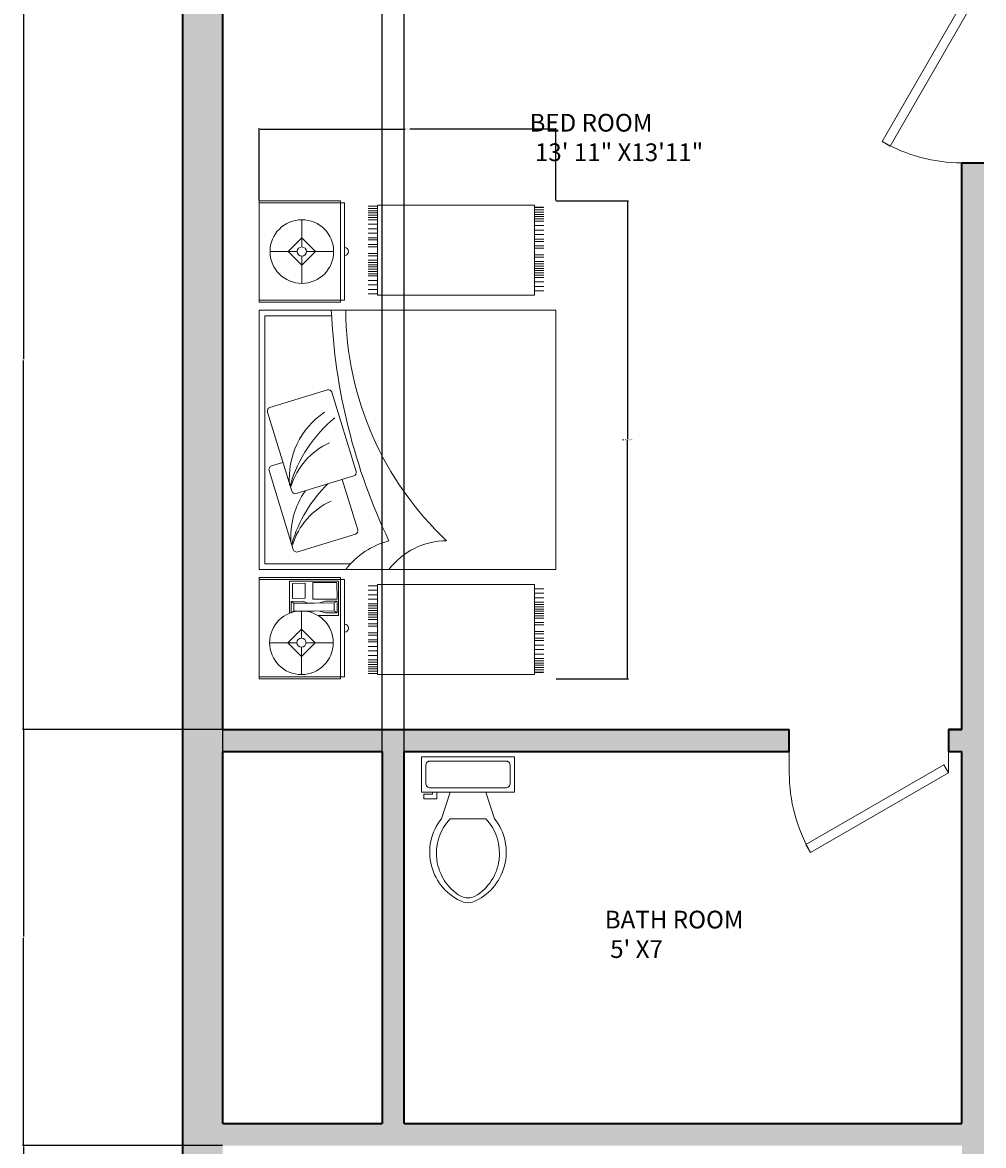
# Model space of a CAD drawing. Units: inches. Extents: x -29 to 404, y -32 to 761.
# Tile 3 of 5: x -29 to 189, y 193 to 447. Entities that reach past the tile are written whole.
import ezdxf

# ---------------------------------------------------------------- set-up
doc = ezdxf.new("R2010")
doc.units = ezdxf.units.IN
doc.header["$MEASUREMENT"] = 0
for name, color, linetype, lineweight in [('A-ANNO-DIMS', 2, 'Continuous', 18), ('A-AREA-IDEN', 7, 'Continuous', 18), ('A-FLOR-FIXT', 9, 'Continuous', 18), ('A-FURN', 8, 'Continuous', 18), ('A-WALL', 7, 'Continuous', 35), ('doors', 40, 'Continuous', 20)]:
    doc.layers.add(name, color=color, linetype=linetype, lineweight=lineweight)
doc.layers.add('A-WALL-PATT', color=251, linetype='Continuous', lineweight=13, true_color=0x636466)
doc.styles.get("Standard").update_dxf_attribs({"font": 'arial.ttf'})
doc.dimstyles.get("Standard").update_dxf_attribs({"dimtxt": 0.18, "dimasz": 0.18, "dimexe": 0.18, "dimexo": 0.0625, "dimgap": 0.09, "dimtad": 0, "dimtih": 1, "dimtoh": 1, "dimdec": 4, "dimzin": 0, "dimdsep": 46, "dimtxsty": 'Standard', "dimcen": 0.09, "dimadec": 0, "dimazin": 0, "dimtfac": 1, "dimtdec": 4, "dimtofl": 0, "dimtmove": 0, "dimatfit": 3, "dimfxl": 1, "dimtolj": 1, "dimtzin": 0, "dimarcsym": 0})

# ---------------------------------------------------------------- blocks, each defined once
blk = doc.blocks.new('3')
for p, q in [((185.8665, 224.6766), (185.8665, 225.2363)), ((185.8665, 225.2363), (186.566, 225.2363)), ((185.8805, 224.6487), (185.8805, 225.2363)), ((186.552, 225.2363), (186.552, 224.6487)), ((186.566, 225.2363), (186.566, 224.6766)), ((186.6199, 225.2363), (186.6199, 224.6399)), ((188.4089, 225.2363), (186.6199, 225.2363)), ((188.4089, 224.7393), (188.4089, 225.2363)), ((188.4627, 225.2363), (188.4627, 224.6766)), ((189.1623, 225.2363), (188.4627, 225.2363)), ((188.4767, 225.2363), (188.4767, 224.6486)), ((189.1483, 224.6486), (189.1483, 225.2363)), ((189.1623, 224.6766), (189.1623, 225.2363)), ((186.1157, 225.1643), (186.1157, 224.9763)), ((187.3034, 225.1683), (186.7581, 225.0015)), ((187.7059, 225.1793), (187.1607, 225.0124)), ((187.3344, 225.1518), (187.3586, 225.073)), ((187.737, 225.1628), (187.8585, 224.7657)), ((188.8125, 225.1618), (188.8125, 224.9738)), ((186.0216, 224.9449), (186.1157, 225.0389)), ((186.1157, 225.0389), (186.2097, 224.9449)), ((186.5397, 225.0274), (186.3193, 225.0266)), ((186.3215, 225.0167), (186.4008, 225.017)), ((186.3334, 224.9969), (186.3215, 225.0167)), ((186.3334, 224.9969), (186.389, 224.9971)), ((186.334, 224.858), (186.3334, 224.9969)), ((186.4008, 225.017), (186.389, 224.9971)), ((186.3895, 224.8582), (186.389, 224.9971)), ((186.4008, 225.017), (186.4011, 224.9376)), ((186.5409, 224.6901), (186.5397, 225.0274)), ((188.8125, 225.0365), (188.7185, 224.9424)), ((188.9065, 224.9424), (188.8125, 225.0365)), ((186.0843, 224.9449), (185.8963, 224.9449)), ((186.1157, 224.8509), (186.0216, 224.9449)), ((186.2097, 224.9449), (186.1157, 224.8509)), ((186.1157, 224.9136), (186.1157, 224.7256)), ((186.147, 224.9449), (186.335, 224.9449)), ((186.4011, 224.9376), (186.3894, 224.8979)), ((186.7416, 224.9704), (186.8631, 224.5734)), ((187.1442, 224.9814), (187.2657, 224.5843)), ((188.7812, 224.9424), (188.5931, 224.9424)), ((188.7185, 224.9424), (188.8125, 224.8484)), ((188.8125, 224.8484), (188.9065, 224.9424)), ((188.8125, 224.9111), (188.8125, 224.723)), ((188.8438, 224.9424), (189.0319, 224.9424)), ((186.3023, 224.8297), (186.3029, 224.6892)), ((186.3314, 224.9055), (186.3338, 224.8977)), ((186.334, 224.858), (186.3345, 224.7191)), ((186.3895, 224.8582), (186.39, 224.7193)), ((186.3224, 224.7786), (186.3341, 224.8183)), ((186.3227, 224.6992), (186.3224, 224.7786)), ((186.4017, 224.7789), (186.3897, 224.8185)), ((186.402, 224.6995), (186.4017, 224.7789)), ((186.566, 224.6766), (185.8665, 224.6766)), ((186.3029, 224.6892), (186.5409, 224.6901)), ((186.3345, 224.7191), (186.3227, 224.6992)), ((186.3227, 224.6992), (186.402, 224.6995)), ((186.3345, 224.7191), (186.39, 224.7193)), ((186.402, 224.6995), (186.39, 224.7193)), ((187.842, 224.7347), (187.2967, 224.5678)), ((188.4089, 224.7393), (188.4089, 223.1907)), ((188.4627, 224.6766), (189.1623, 224.6766)), ((186.552, 224.6487), (185.8805, 224.6487)), ((186.6199, 224.6399), (186.6199, 223.1907)), ((187.2416, 224.6632), (186.8942, 224.5569)), ((188.4767, 224.6486), (189.1483, 224.6486)), ((185.904, 224.4849, -0.9094), (185.904, 224.4204, -0.9094)), ((185.9195, 224.4849, -0.9094), (185.9195, 224.4204, -0.9094)), ((185.9195, 224.4849, -0.9094), (185.9195, 224.4204, -0.9094)), ((185.935, 224.4849, -0.9094), (185.935, 224.4204, -0.9094)), ((185.9505, 224.4849, -0.9094), (185.9505, 224.4204, -0.9094)), ((185.966, 224.4849, -0.9094), (185.966, 224.4204, -0.9094)), ((185.9815, 224.4849, -0.9094), (185.9815, 224.4204, -0.9094)), ((185.997, 224.4849, -0.9094), (185.997, 224.4204, -0.9094)), ((186.028, 224.4849, -0.9094), (186.028, 224.4204, -0.9094)), ((186.059, 224.4849, -0.9094), (186.059, 224.4204, -0.9094)), ((186.09, 224.4849, -0.9094), (186.09, 224.4204, -0.9094)), ((186.09, 224.4849, -0.9094), (186.09, 224.4204, -0.9094)), ((186.121, 224.4849, -0.9094), (186.121, 224.4204, -0.9094)), ((186.1365, 224.4849, -0.9094), (186.1365, 224.4204, -0.9094)), ((186.1675, 224.4849, -0.9094), (186.1675, 224.4204, -0.9094)), ((186.183, 224.4849, -0.9094), (186.183, 224.4204, -0.9094)), ((186.2295, 224.4849, -0.9094), (186.2295, 224.4204, -0.9094)), ((186.245, 224.4849, -0.9094), (186.245, 224.4204, -0.9094)), ((186.276, 224.4849, -0.9094), (186.276, 224.4204, -0.9094)), ((186.2915, 224.4849, -0.9094), (186.2915, 224.4204, -0.9094)), ((186.307, 224.4849, -0.9094), (186.307, 224.4204, -0.9094)), ((186.3225, 224.4849, -0.9094), (186.3225, 224.4204, -0.9094)), ((186.338, 224.4849, -0.9094), (186.338, 224.4204, -0.9094)), ((186.3535, 224.4849, -0.9094), (186.3535, 224.4204, -0.9094)), ((186.369, 224.4849, -0.9094), (186.369, 224.4204, -0.9094)), ((186.3845, 224.4849, -0.9094), (186.3845, 224.4204, -0.9094)), ((186.4155, 224.4849, -0.9094), (186.4155, 224.4204, -0.9094)), ((186.4465, 224.4849, -0.9094), (186.4465, 224.4204, -0.9094)), ((186.4775, 224.4849, -0.9094), (186.4775, 224.4204, -0.9094)), ((186.5085, 224.4849, -0.9094), (186.5085, 224.4204, -0.9094)), ((188.5202, 224.4849, -0.9094), (188.5202, 224.4204, -0.9094)), ((188.5512, 224.4849, -0.9094), (188.5512, 224.4204, -0.9094)), ((188.5822, 224.4849, -0.9094), (188.5822, 224.4204, -0.9094)), ((188.6132, 224.4849, -0.9094), (188.6132, 224.4204, -0.9094)), ((188.6442, 224.4849, -0.9094), (188.6442, 224.4204, -0.9094)), ((188.6597, 224.4849, -0.9094), (188.6597, 224.4204, -0.9094)), ((188.6752, 224.4849, -0.9094), (188.6752, 224.4204, -0.9094)), ((188.6907, 224.4849, -0.9094), (188.6907, 224.4204, -0.9094)), ((188.7062, 224.4849, -0.9094), (188.7062, 224.4204, -0.9094)), ((188.7217, 224.4849, -0.9094), (188.7217, 224.4204, -0.9094)), ((188.7372, 224.4849, -0.9094), (188.7372, 224.4204, -0.9094)), ((188.7527, 224.4849, -0.9094), (188.7527, 224.4204, -0.9094)), ((188.7837, 224.4849, -0.9094), (188.7837, 224.4204, -0.9094)), ((188.7992, 224.4849, -0.9094), (188.7992, 224.4204, -0.9094)), ((188.8457, 224.4849, -0.9094), (188.8457, 224.4204, -0.9094)), ((188.8612, 224.4849, -0.9094), (188.8612, 224.4204, -0.9094)), ((188.8922, 224.4849, -0.9094), (188.8922, 224.4204, -0.9094)), ((188.9077, 224.4849, -0.9094), (188.9077, 224.4204, -0.9094)), ((188.9387, 224.4849, -0.9094), (188.9387, 224.4204, -0.9094)), ((188.9387, 224.4849, -0.9094), (188.9387, 224.4204, -0.9094)), ((188.9697, 224.4849, -0.9094), (188.9697, 224.4204, -0.9094)), ((189.0007, 224.4849, -0.9094), (189.0007, 224.4204, -0.9094)), ((189.0317, 224.4849, -0.9094), (189.0317, 224.4204, -0.9094)), ((189.0472, 224.4849, -0.9094), (189.0472, 224.4204, -0.9094)), ((189.0627, 224.4849, -0.9094), (189.0627, 224.4204, -0.9094)), ((189.0782, 224.4849, -0.9094), (189.0782, 224.4204, -0.9094)), ((189.0937, 224.4849, -0.9094), (189.0937, 224.4204, -0.9094)), ((189.1092, 224.4849, -0.9094), (189.1092, 224.4204, -0.9094)), ((189.1092, 224.4849, -0.9094), (189.1092, 224.4204, -0.9094)), ((189.1247, 224.4849, -0.9094), (189.1247, 224.4204, -0.9094)), ((185.8974, 224.4204, -0.9094), (185.8974, 223.3378, -0.9094)), ((185.8974, 224.4204, -0.9094), (186.5174, 224.4204, -0.9094)), ((186.5174, 224.4204, -0.9094), (186.5174, 223.3378, -0.9094)), ((189.1313, 224.4204, -0.9094), (188.5113, 224.4204, -0.9094)), ((188.5113, 224.4204, -0.9094), (188.5113, 223.3378, -0.9094)), ((189.1313, 224.4204, -0.9094), (189.1313, 223.3378, -0.9094)), ((185.8974, 223.3378, -0.9094), (186.5174, 223.3378, -0.9094)), ((185.9114, 223.3378, -0.9094), (185.9114, 223.2789, -0.9094)), ((185.9114, 223.3378, -0.9094), (185.9114, 223.2789, -0.9094)), ((185.9114, 223.3378, -0.9094), (185.9114, 223.2789, -0.9094)), ((185.9138, 223.3378, -0.9094), (185.9138, 223.2732, -0.9094)), ((185.9293, 223.3378, -0.9094), (185.9293, 223.2732, -0.9094)), ((185.9293, 223.3378, -0.9094), (185.9293, 223.2732, -0.9094)), ((185.9448, 223.3378, -0.9094), (185.9448, 223.2732, -0.9094)), ((185.9603, 223.3378, -0.9094), (185.9603, 223.2732, -0.9094)), ((185.9758, 223.3378, -0.9094), (185.9758, 223.2732, -0.9094)), ((185.9913, 223.3378, -0.9094), (185.9913, 223.2732, -0.9094)), ((186.0068, 223.3378, -0.9094), (186.0068, 223.2732, -0.9094)), ((186.0378, 223.3378, -0.9094), (186.0378, 223.2732, -0.9094)), ((186.0688, 223.3378, -0.9094), (186.0688, 223.2732, -0.9094)), ((186.0998, 223.3378, -0.9094), (186.0998, 223.2732, -0.9094)), ((186.0998, 223.3378, -0.9094), (186.0998, 223.2732, -0.9094)), ((186.1308, 223.3378, -0.9094), (186.1308, 223.2732, -0.9094)), ((186.1463, 223.3378, -0.9094), (186.1463, 223.2732, -0.9094)), ((186.1773, 223.3378, -0.9094), (186.1773, 223.2732, -0.9094)), ((186.1928, 223.3378, -0.9094), (186.1928, 223.2732, -0.9094)), ((186.2393, 223.3378, -0.9094), (186.2393, 223.2732, -0.9094)), ((186.2548, 223.3378, -0.9094), (186.2548, 223.2732, -0.9094)), ((186.2858, 223.3378, -0.9094), (186.2858, 223.2732, -0.9094)), ((186.3013, 223.3378, -0.9094), (186.3013, 223.2732, -0.9094)), ((186.3168, 223.3378, -0.9094), (186.3168, 223.2732, -0.9094)), ((186.3323, 223.3378, -0.9094), (186.3323, 223.2732, -0.9094)), ((186.3478, 223.3378, -0.9094), (186.3478, 223.2732, -0.9094)), ((186.3633, 223.3378, -0.9094), (186.3633, 223.2732, -0.9094)), ((186.3788, 223.3378, -0.9094), (186.3788, 223.2732, -0.9094)), ((186.3943, 223.3378, -0.9094), (186.3943, 223.2732, -0.9094)), ((186.4253, 223.3378, -0.9094), (186.4253, 223.2732, -0.9094)), ((186.4563, 223.3378, -0.9094), (186.4563, 223.2732, -0.9094)), ((186.4873, 223.3378, -0.9094), (186.4873, 223.2732, -0.9094)), ((189.1313, 223.3378, -0.9094), (188.5113, 223.3378, -0.9094)), ((188.5414, 223.3378, -0.9094), (188.5414, 223.2732, -0.9094)), ((188.5724, 223.3378, -0.9094), (188.5724, 223.2732, -0.9094)), ((188.6034, 223.3378, -0.9094), (188.6034, 223.2732, -0.9094)), ((188.6344, 223.3378, -0.9094), (188.6344, 223.2732, -0.9094)), ((188.6499, 223.3378, -0.9094), (188.6499, 223.2732, -0.9094)), ((188.6654, 223.3378, -0.9094), (188.6654, 223.2732, -0.9094)), ((188.6809, 223.3378, -0.9094), (188.6809, 223.2732, -0.9094)), ((188.6964, 223.3378, -0.9094), (188.6964, 223.2732, -0.9094)), ((188.7119, 223.3378, -0.9094), (188.7119, 223.2732, -0.9094)), ((188.7274, 223.3378, -0.9094), (188.7274, 223.2732, -0.9094)), ((188.7429, 223.3378, -0.9094), (188.7429, 223.2732, -0.9094)), ((188.7739, 223.3378, -0.9094), (188.7739, 223.2732, -0.9094)), ((188.7894, 223.3378, -0.9094), (188.7894, 223.2732, -0.9094)), ((188.8359, 223.3378, -0.9094), (188.8359, 223.2732, -0.9094)), ((188.8514, 223.3378, -0.9094), (188.8514, 223.2732, -0.9094)), ((188.8824, 223.3378, -0.9094), (188.8824, 223.2732, -0.9094)), ((188.8979, 223.3378, -0.9094), (188.8979, 223.2732, -0.9094)), ((188.9289, 223.3378, -0.9094), (188.9289, 223.2732, -0.9094)), ((188.9289, 223.3378, -0.9094), (188.9289, 223.2732, -0.9094)), ((188.9599, 223.3378, -0.9094), (188.9599, 223.2732, -0.9094)), ((188.9909, 223.3378, -0.9094), (188.9909, 223.2732, -0.9094)), ((189.022, 223.3378, -0.9094), (189.022, 223.2732, -0.9094)), ((189.0375, 223.3378, -0.9094), (189.0375, 223.2732, -0.9094)), ((189.053, 223.3378, -0.9094), (189.053, 223.2732, -0.9094)), ((189.0685, 223.3378, -0.9094), (189.0685, 223.2732, -0.9094)), ((189.084, 223.3378, -0.9094), (189.084, 223.2732, -0.9094)), ((189.0995, 223.3378, -0.9094), (189.0995, 223.2732, -0.9094)), ((189.0995, 223.3378, -0.9094), (189.0995, 223.2732, -0.9094)), ((189.115, 223.3378, -0.9094), (189.115, 223.2732, -0.9094)), ((189.1173, 223.3378, -0.9094), (189.1173, 223.2789, -0.9094)), ((189.1173, 223.3378, -0.9094), (189.1173, 223.2789, -0.9094)), ((189.1173, 223.3378, -0.9094), (189.1173, 223.2789, -0.9094)), ((186.6199, 223.1907), (188.4089, 223.1907))]:
    blk.add_line(p, q)
blk.add_lwpolyline([(188.3691, 224.7374), (188.3691, 225.1965), (186.6596, 225.1965), (186.6596, 224.606)])
for points in [[(186.4217, 225.0072), (186.422, 224.9199), (186.5252, 224.9202), (186.5249, 225.0075)], [(186.4153, 224.8663), (186.4159, 224.6996), (186.531, 224.7), (186.5304, 224.8667)]]:
    blk.add_lwpolyline(points, close=True)
for points in [[(186.6199, 224.6399, -0.162278), (186.8186, 224.3418, -0.100664), (188.4089, 224.7393, -0.100664)], [(186.6199, 224.3418, -0.236068), (186.8186, 223.9442, -0.205258), (188.4089, 224.6399, -0.205258)]]:
    blk.add_lwpolyline(points, format="xyb")
for centre, radius in [((186.1157, 224.9449), 0.2194), ((188.8125, 224.9424), 0.2194), ((186.1157, 224.9449), 0.0313), ((188.8125, 224.9424), 0.0313)]:
    blk.add_circle(centre, radius)
for centre, radius, start, end in [((187.3107, 225.1446), 0.0248, 17.0142, 107.0142), ((187.7132, 225.1555), 0.0248, 17.0142, 107.0142), ((186.7654, 224.9777), 0.0248, 107.0142, 197.0142), ((186.6474, 224.5408), 0.4873, 24.22087, 73.06906), ((186.8477, 224.4712), 0.5468, 54.68511, 95.16051), ((186.5359, 224.1054), 0.9426, 44.27274, 73.71889), ((187.1679, 224.9887), 0.0248, 107.0142, 197.0142), ((187.0499, 224.5517), 0.4873, 24.22087, 73.06906), ((187.2502, 224.4821), 0.5468, 33.78007, 95.16051), ((186.9385, 224.1164), 0.9426, 39.40233, 73.71889), ((187.8347, 224.7585), 0.0248, 287.0142, 17.0142), ((186.2163, 224.6487), 0.028, 180, 0), ((188.8125, 224.6486), 0.028, 180, 0), ((186.8869, 224.5806), 0.0248, 197.0142, 287.0142), ((187.2894, 224.5916), 0.0248, 197.0142, 287.0142)]:
    blk.add_arc(centre, radius, start, end)
blk = doc.blocks.new('Toilet - top')
for p, q in [((9.5, -6), (9.5, -2)), ((-10, -8.5), (-8, -8.5)), ((-10, -9.5), (-10, -8.5)), ((-7, -9.5), (-10, -9.5)), ((-8, -8.5), (-8, -8)), ((-7, -8), (-7, -9.5)), ((-4, -8), (-6, -14)), ((4, -8), (6, -14)), ((4, -14), (-4, -14))]:
    blk.add_line(p, q)
blk.add_lwpolyline([(10.5, -8), (10.5, 0), (-10.5, 0), (-10.5, -8)], close=True)
for points in [[(-9.5, -2), (-9.5, -6)], [(8.5, -1), (-8.5, -1)], [(-8.5, -7), (8.5, -7)]]:
    blk.add_lwpolyline(points)
for centre, radius, start, end in [((-8.62, -1.88), 0.884, 81.8699, 188.1301), ((8.62, -1.88), 0.884, 351.8699, 98.1301), ((-8.62, -6.12), 0.884, 171.8699, 278.1301), ((8.62, -6.12), 0.884, 261.8699, 8.1301), ((3.52, -21.58), 12.17, 141.4691, 247.9714), ((4.2, -21.82), 11.33, 136.3677, 238.9468), ((-3.52, -21.58), 12.17, 292.0284, 38.5307), ((-4.2, -21.82), 11.33, 301.053, 43.6321), ((0, -27.88), 4, 245.7318, 294.2682), ((0, -29), 4, 254.8605, 285.1395)]:
    blk.add_arc(centre, radius, start, end)
blk = doc.blocks.new('*U6')
for p, q in [((0, 0), (0, -100)), ((750, 0), (750, -100))]:
    blk.add_line(p, q)
blk.add_lwpolyline([(0, 0), (649.5, 375), (671.4, 337.1), (21.9, -37.9)], close=True)
blk.add_arc((0, 0), 750, 0, 30)
blk = doc.blocks.new('*U7')
for p, q in [((0, 0), (0, 100)), ((750, 0), (750, 100))]:
    blk.add_line(p, q)
blk.add_lwpolyline([(0, 0), (649.5, -375), (671.4, -337.1), (21.9, 37.9)], close=True)
blk.add_arc((0, 0), 750, 330, 0)
blk = doc.blocks.new('*D13')
at = {"layer": 'A-ANNO-DIMS', "color": 0, "lineweight": -2, "transparency": 16777216}
for p, q in [((92.01, 406.85), (108.33, 406.85)), ((108.15, 406.67), (108.15, 353.04)), ((108.15, 299.03), (108.15, 352.67)), ((92.01, 298.85), (108.33, 298.85))]:
    blk.add_line(p, q, dxfattribs=at)
at = {"layer": 'A-ANNO-DIMS', "color": 0, "transparency": 16777216}
for points in [[(108.12, 406.67), (108.18, 406.67), (108.15, 406.85)], [(108.12, 299.03), (108.18, 299.03), (108.15, 298.85)]]:
    blk.add_solid(points, dxfattribs=at)
at = {"layer": 'Defpoints', "color": 0, "transparency": 16777216}
for p in [(91.95, 406.85), (108.15, 406.85), (91.95, 298.85)]:
    blk.add_point(p, dxfattribs=at)
at = {"layer": 'A-ANNO-DIMS', "color": 0, "transparency": 16777216, "insert": (108.15, 352.85), "char_height": 0.18, "attachment_point": 5}
blk.add_mtext('\\A1;BED GROUP 108 TYP.', dxfattribs=at)
blk = doc.blocks.new('*D14')
at = {"layer": 'A-ANNO-DIMS', "color": 0, "lineweight": -2, "transparency": 16777216}
for p, q in [((24.92, 406.91), (24.92, 423.23)), ((25.1, 423.05), (57.91, 423.05)), ((91.77, 423.05), (58.96, 423.05)), ((91.95, 406.91), (91.95, 423.23))]:
    blk.add_line(p, q, dxfattribs=at)
at = {"layer": 'A-ANNO-DIMS', "color": 0, "transparency": 16777216}
for points in [[(25.1, 423.08), (25.1, 423.02), (24.92, 423.05)], [(91.77, 423.08), (91.77, 423.02), (91.95, 423.05)]]:
    blk.add_solid(points, dxfattribs=at)
at = {"layer": 'Defpoints', "color": 0, "transparency": 16777216}
for p in [(24.92, 423.05), (24.92, 406.85), (91.95, 406.85)]:
    blk.add_point(p, dxfattribs=at)
at = {"layer": 'A-ANNO-DIMS', "color": 0, "transparency": 16777216, "insert": (58.44, 423.05), "char_height": 0.18, "attachment_point": 5}
blk.add_mtext('\\A1;67 TYP.', dxfattribs=at)
blk = doc.blocks.new('*D33')
at = {"layer": 'A-ANNO-DIMS', "color": 0, "lineweight": -2, "transparency": 16777216}
for p, q in [((16.62, 193.43), (-28.55, 193.43)), ((-28.37, 193.25), (-28.37, 99.12)), ((-28.37, 4.61), (-28.37, 98.75)), ((7.62, 4.43), (-28.55, 4.43))]:
    blk.add_line(p, q, dxfattribs=at)
at = {"layer": 'A-ANNO-DIMS', "color": 0, "transparency": 16777216}
for points in [[(-28.4, 193.25), (-28.34, 193.25), (-28.37, 193.43)], [(-28.4, 4.61), (-28.34, 4.61), (-28.37, 4.43)]]:
    blk.add_solid(points, dxfattribs=at)
at = {"layer": 'Defpoints', "color": 0, "transparency": 16777216}
for p in [(-28.37, 193.43), (16.68, 193.43), (7.68, 4.43)]:
    blk.add_point(p, dxfattribs=at)
at = {"layer": 'A-ANNO-DIMS', "color": 0, "transparency": 16777216, "insert": (-28.37, 98.93), "char_height": 0.18, "attachment_point": 5}
blk.add_mtext('\\A1;189', dxfattribs=at)
blk = doc.blocks.new('*D34')
at = {"layer": 'A-ANNO-DIMS', "color": 0, "lineweight": -2, "transparency": 16777216}
for p, q in [((16.62, 287.43), (-28.55, 287.43)), ((-28.37, 287.25), (-28.37, 240.62)), ((-28.37, 193.61), (-28.37, 240.25)), ((16.62, 193.43), (-28.55, 193.43))]:
    blk.add_line(p, q, dxfattribs=at)
at = {"layer": 'A-ANNO-DIMS', "color": 0, "transparency": 16777216}
for points in [[(-28.4, 287.25), (-28.34, 287.25), (-28.37, 287.43)], [(-28.4, 193.61), (-28.34, 193.61), (-28.37, 193.43)]]:
    blk.add_solid(points, dxfattribs=at)
at = {"layer": 'Defpoints', "color": 0, "transparency": 16777216}
for p in [(-28.37, 287.43), (16.68, 287.43), (16.68, 193.43)]:
    blk.add_point(p, dxfattribs=at)
at = {"layer": 'A-ANNO-DIMS', "color": 0, "transparency": 16777216, "insert": (-28.37, 240.43), "char_height": 0.18, "attachment_point": 5}
blk.add_mtext('\\A1;94', dxfattribs=at)
blk = doc.blocks.new('*D35')
at = {"layer": 'A-ANNO-DIMS', "color": 0, "lineweight": -2, "transparency": 16777216}
for p, q in [((16.62, 454.43), (-28.55, 454.43)), ((-28.37, 454.25), (-28.37, 371.12)), ((-28.37, 287.61), (-28.37, 370.75)), ((16.62, 287.43), (-28.55, 287.43))]:
    blk.add_line(p, q, dxfattribs=at)
at = {"layer": 'A-ANNO-DIMS', "color": 0, "transparency": 16777216}
for points in [[(-28.4, 454.25), (-28.34, 454.25), (-28.37, 454.43)], [(-28.4, 287.61), (-28.34, 287.61), (-28.37, 287.43)]]:
    blk.add_solid(points, dxfattribs=at)
at = {"layer": 'Defpoints', "color": 0, "transparency": 16777216}
for p in [(-28.37, 454.43), (16.68, 454.43), (16.68, 287.43)]:
    blk.add_point(p, dxfattribs=at)
at = {"layer": 'A-ANNO-DIMS', "color": 0, "transparency": 16777216, "insert": (-28.37, 370.93), "char_height": 0.18, "attachment_point": 5}
blk.add_mtext('\\A1;167', dxfattribs=at)
blk = doc.blocks.new('*D59')
at = {"layer": 'A-ANNO-DIMS', "color": 0, "lineweight": -2, "transparency": 16777216}
for p, q in [((16.68, 198.5), (16.68, 760.66)), ((16.86, 760.48), (34.46, 760.48)), ((52.5, 760.48), (34.9, 760.48)), ((52.68, 198.5), (52.68, 760.66))]:
    blk.add_line(p, q, dxfattribs=at)
at = {"layer": 'A-ANNO-DIMS', "color": 0, "transparency": 16777216}
for points in [[(16.86, 760.51), (16.86, 760.45), (16.68, 760.48)], [(52.5, 760.51), (52.5, 760.45), (52.68, 760.48)]]:
    blk.add_solid(points, dxfattribs=at)
at = {"layer": 'Defpoints', "color": 0, "transparency": 16777216}
for p in [(52.68, 760.48), (16.68, 198.43), (52.68, 198.43)]:
    blk.add_point(p, dxfattribs=at)
at = {"layer": 'A-ANNO-DIMS', "color": 0, "transparency": 16777216, "insert": (34.68, 760.48), "char_height": 0.18, "attachment_point": 5}
blk.add_mtext('\\A1;36', dxfattribs=at)
blk = doc.blocks.new('*D60')
at = {"layer": 'A-ANNO-DIMS', "color": 0, "lineweight": -2, "transparency": 16777216}
for p, q in [((52.68, 198.5), (52.68, 760.66)), ((52.86, 760.48), (55.03, 760.48)), ((57.5, 760.48), (55.33, 760.48)), ((57.68, 198.5), (57.68, 760.66))]:
    blk.add_line(p, q, dxfattribs=at)
at = {"layer": 'A-ANNO-DIMS', "color": 0, "transparency": 16777216}
for points in [[(52.86, 760.51), (52.86, 760.45), (52.68, 760.48)], [(57.5, 760.51), (57.5, 760.45), (57.68, 760.48)]]:
    blk.add_solid(points, dxfattribs=at)
at = {"layer": 'Defpoints', "color": 0, "transparency": 16777216}
for p in [(57.68, 760.48), (52.68, 198.43), (57.68, 198.43)]:
    blk.add_point(p, dxfattribs=at)
at = {"layer": 'A-ANNO-DIMS', "color": 0, "transparency": 16777216, "insert": (55.18, 760.48), "char_height": 0.18, "attachment_point": 5}
blk.add_mtext('\\A1;5', dxfattribs=at)

msp = doc.modelspace()

# ---------------------------------------------------------------- hatches: boundary and pattern name
at = {"layer": 'A-WALL-PATT'}
h = msp.add_hatch(color=256, dxfattribs=at)
h.dxf.hatch_style = 1
h.paths.add_polyline_path([(188.678, 415.434), (183.678, 415.434), (183.678, 287.434), (180.678, 287.434), (180.678, 282.434), (183.678, 282.434), (183.678, 198.434), (57.678, 198.434), (57.678, 282.434), (144.678, 282.434), (144.678, 287.434), (16.678, 287.434), (16.678, 548.434), (144.678, 548.434, -0.1168354), (148.504, 564.585), (148.451, 564.616), (149.501, 566.434), (180.678, 548.434), (180.678, 543.434), (183.678, 543.434), (191.678, 543.434), (191.678, 548.434), (191.678, 553.634), (225.453, 573.134), (226.591, 571.164), (226.533, 571.131, -0.1168354), (230.678, 553.634), (230.678, 548.434), (358.678, 548.434), (358.678, 471.434), (322.678, 471.434), (322.678, 543.434), (358.678, 543.434), (358.678, 548.434), (230.678, 548.434), (230.678, 543.434), (233.678, 543.434), (252.678, 543.434), (252.678, 466.434), (260.678, 466.434), (260.678, 471.434), (257.678, 471.434), (257.678, 543.434), (317.678, 543.434), (317.678, 471.434), (296.678, 471.434), (296.678, 466.434), (358.678, 466.434), (358.678, 198.434), (286.678, 198.434), (286.678, 193.434), (358.678, 193.434), (358.678, 97.434), (238.678, 97.434), (238.678, 193.434), (250.678, 193.434), (250.678, 198.434), (233.678, 198.434), (233.678, 92.434), (358.678, 92.434), (358.678, 13.434), (296.678, 13.434), (296.678, 4.434), (367.678, 4.434), (367.678, 724.434), (7.678, 724.434), (7.678, 4.434), (188.678, 4.434), (188.678, 13.434), (188.678, 154.434), (183.678, 154.434), (183.678, 13.434), (49.651, 13.434), (48.286, 12.069), (46.92, 13.434), (16.678, 13.434), (16.678, 193.434), (183.678, 193.434), (183.678, 190.434), (188.678, 190.434)])
h.paths.add_polyline_path([(52.678, 282.434), (52.678, 198.434), (16.678, 198.434), (16.678, 282.434)], flags=16)

# ---------------------------------------------------------------- linework, layer by layer
at = {"layer": 'A-WALL'}
for p, q in [((16.678, 287.434), (16.678, 715.434)), ((183.678, 287.434), (183.678, 415.434)), ((183.678, 415.434), (188.678, 415.434)), ((16.678, 287.434), (144.678, 287.434)), ((144.678, 282.434), (144.678, 287.434)), ((180.678, 287.434), (183.678, 287.434)), ((183.678, 287.434), (180.678, 287.434)), ((180.678, 287.434), (180.678, 282.434)), ((16.678, 282.434), (52.678, 282.434)), ((16.678, 198.434), (16.678, 282.434)), ((16.678, 282.434), (52.678, 282.434)), ((52.678, 282.434), (52.678, 198.434)), ((57.678, 282.434), (144.678, 282.434)), ((57.678, 198.434), (57.678, 282.434)), ((180.678, 282.434), (183.678, 282.434)), ((183.678, 198.434), (183.678, 282.434)), ((16.678, 198.434), (52.678, 198.434)), ((57.678, 198.434), (183.678, 198.434))]:
    msp.add_line(p, q, dxfattribs=at)
msp.add_lwpolyline([(188.678, 4.434), (7.678, 4.434), (7.678, 724.434), (367.678, 724.434), (367.678, 4.434), (296.678, 4.434)], dxfattribs=at)

# ---------------------------------------------------------------- block references
at = {"layer": 'A-FLOR-FIXT'}
msp.add_blockref('Toilet - top', (72.088, 281.271), dxfattribs=at)
at = {"layer": 'A-FURN', "xscale": 32.76894482774335, "yscale": 32.76894482774335, "zscale": 32.76894482774335, "rotation": 89.99999999999999}
msp.add_blockref('3', (7405.674, -5791.797), dxfattribs=at)
at = {"layer": 'doors', "xscale": 0.0479999999999998, "yscale": 0.0479999999999998, "zscale": 0.0479999999999998}
for name, p, rotation in [('*U7', (183.678, 451.434), 270), ('*U6', (180.678, 277.634), 180)]:
    msp.add_blockref(name, p, dxfattribs=dict(at, rotation=rotation))

# ---------------------------------------------------------------- texts
at = {"layer": 'A-AREA-IDEN', "char_height": 4, "attachment_point": 1}
for s, width, insert in [('BED ROOM\\P 13\' 11" X13\'11"', 80.5, (85.992, 426.479)), ("BATH ROOM\\P 5' X7", 60, (102.992, 246.479))]:
    msp.add_mtext_dynamic_manual_height_columns(s, width=width, gutter_width=1, heights=[0], dxfattribs=dict(at, insert=insert))

# ---------------------------------------------------------------- dimensions: what is measured, and where the dimension line sits
at = {"layer": 'A-ANNO-DIMS'}
for base, p1, p2, picture, middle in [((52.678, 760.484), (16.678, 198.434), (52.678, 198.434), '*D59', (34.678, 760.484)), ((57.678, 760.484), (52.678, 198.434), (57.678, 198.434), '*D60', (55.178, 760.484))]:
    dim = msp.add_linear_dim(base=base, p1=p1, p2=p2, dimstyle='Standard', override={"dimdec": 0, "dimlfac": 1, "dimrnd": 0, "dimzin": 0, "dimdsep": 46, "dimlunit": 2}, dxfattribs=at)
    dim.commit()
    dim.dimension.update_dxf_attribs({"geometry": picture, "text_midpoint": middle})
for base, p1, p2, picture, middle in [((-28.372, 454.434), (16.678, 287.434), (16.678, 454.434), '*D35', (-28.372, 370.934)), ((-28.372, 287.434), (16.678, 193.434), (16.678, 287.434), '*D34', (-28.372, 240.434)), ((-28.372, 193.434), (7.678, 4.434), (16.678, 193.434), '*D33', (-28.372, 98.934))]:
    dim = msp.add_linear_dim(base=base, p1=p1, p2=p2, angle=90, dimstyle='Standard', override={"dimdec": 0, "dimlfac": 1, "dimrnd": 0, "dimzin": 0, "dimdsep": 46, "dimlunit": 2}, dxfattribs=at)
    dim.commit()
    dim.dimension.update_dxf_attribs({"geometry": picture, "text_midpoint": middle})
for base, p1, p2, angle, text, picture, middle in [((24.919, 423.052), (91.951, 406.852), (24.919, 406.852), 180, '<> TYP.', '*D14', (58.435, 423.052)), ((108.151, 406.852), (91.951, 298.852), (91.951, 406.852), 90, 'BED GROUP <> TYP.', '*D13', (108.151, 352.852))]:
    dim = msp.add_linear_dim(base=base, p1=p1, p2=p2, angle=angle, text=text, dimstyle='Standard', override={"dimdec": 0, "dimlfac": 1, "dimrnd": 0, "dimzin": 0, "dimdsep": 46, "dimlunit": 2}, dxfattribs=at)
    dim.commit()
    dim.dimension.update_dxf_attribs({"geometry": picture, "text_midpoint": middle})

doc.saveas('drawing.dxf')
